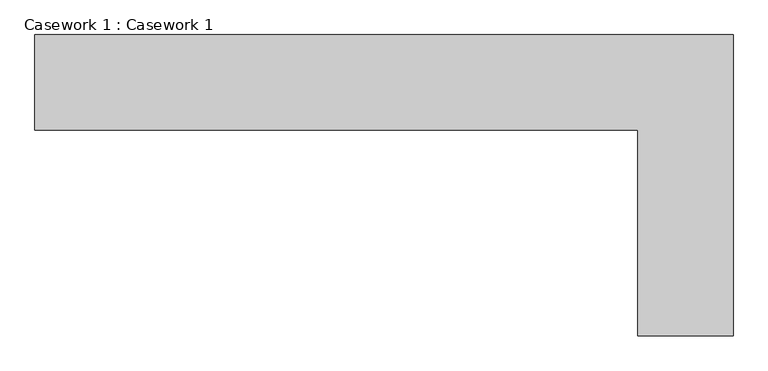
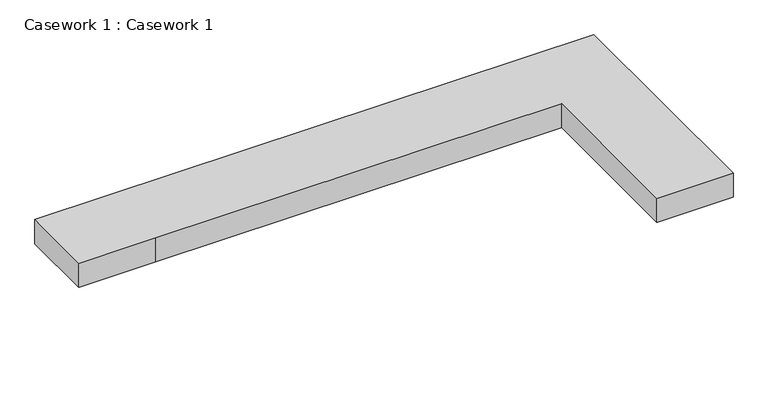
"""IFC4 building model written with IfcOpenShell, lengths in millimetres: furniture geometry, Casework 1 : Casework 1."""

from ifc_helpers import new_model, si_unit, frame, origin, place, context, project, spatial, polyline, outline, extrude, source, transform, mapped, element, save


def casework_1_casework_1_03657681(model_context):
    return source(origin(), model_context, "Body", "SweptSolid", [
        extrude(outline(polyline([(3707.3465688, 11245.3352197), (3707.3465688, 9797.5352197), (3250.1465688, 9797.5352197), (3250.1465688, 10788.1352197), (811.7465688, 10788.1352197), (354.5465688, 10788.1352197), (354.5465688, 11245.3352197), (3707.3465688, 11245.3352197)])), frame((0.0, 0.0, 1219.2), z_axis=(0.0, 0.0, 1.0), x_axis=(1.0, 0.0, 0.0)), (0.0, 0.0, 1.0), 152.4),
    ])


if __name__ == "__main__":
    model = new_model("IFC4")
    model_context = context("Model", 3, world=origin())
    ifc_project = project(units=[si_unit("LENGTHUNIT", "METRE", prefix="MILLI")], contexts=[model_context])
    site = spatial("IfcSite", under=ifc_project)
    building = spatial("IfcBuilding", under=site)
    placement = place(None, origin())
    casework_1_casework_1_shape = casework_1_casework_1_03657681(model_context)
    element("IfcFurniture", 1, ObjectType="Casework 1 : Casework 1", at=placement, inside=building, context=model_context, shape_type="MappedRepresentation", body=[
        mapped(casework_1_casework_1_shape, transform((0.0, 0.0, 0.0), x_axis=(1.0, 0.0, 0.0), y_axis=(0.0, 1.0, 0.0), z_axis=(0.0, 0.0, 1.0))),
    ])
    save(model, "model.ifc")
